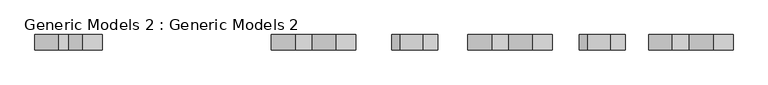
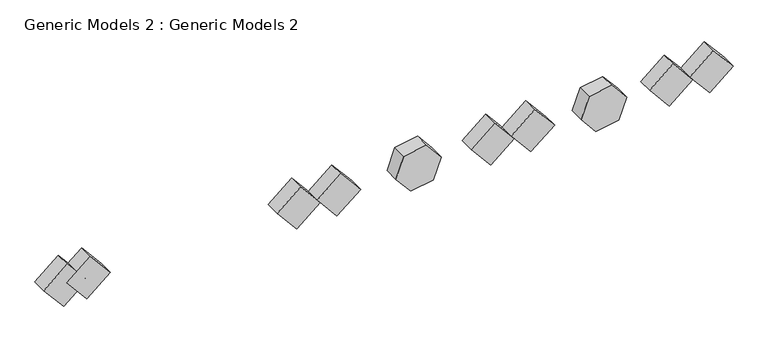
"""IFC4 building model written with IfcOpenShell, lengths in millimetres: proxy geometry, Generic Models 2 : Generic Models 2."""

from ifc_helpers import new_model, si_unit, frame, origin, place, context, project, spatial, polyline, outline, extrude, source, transform, mapped, element, save


def generic_models_2_generic_models_2_4ba01f5b(model_context):
    return source(origin(), model_context, "Body", "SweptSolid", [
        extrude(outline(polyline([(809.5637525, 10146.4778679), (1159.7992719, 9852.5953728), (1080.407325, 9402.3412681), (650.7798588, 9245.9696586), (300.5443394, 9539.8521537), (379.9362862, 9990.1062584), (809.5637525, 10146.4778679)])), frame((0.0, -2288.404596, 0.0), z_axis=(0.0, 1.0, 0.0), x_axis=(0.0, 0.0, 1.0)), (0.0, 0.0, 1.0), 304.8),
        extrude(outline(polyline([(840.3090419, 6475.3232534), (1190.5445612, 6181.4407582), (1111.1526144, 5731.1866535), (681.5251482, 5574.815044), (331.2896288, 5868.6975392), (410.6815756, 6318.9516438), (840.3090419, 6475.3232534)])), frame((0.0, -2288.404596, 0.0), z_axis=(0.0, 1.0, 0.0), x_axis=(0.0, 0.0, 1.0)), (0.0, 0.0, 1.0), 304.8),
        extrude(outline(polyline([(0.0, -609.5999999), (0.0, 0.0), (304.8, 0.0), (304.8, -609.5999999), (0.0, -609.5999999)])), frame((-553.9885527, -2288.404596, 325.3979045), z_axis=(-0.6427876096865387, 0.0, 0.7660444431189787), x_axis=(0.0, 1.0, 0.0)), (0.0, 0.0, 1.0), 609.6),
        extrude(outline(polyline([(0.0, -609.5999999), (0.0, 0.0), (304.8, 0.0), (304.8, -609.5999999), (0.0, -609.5999999)])), frame((-1011.1885527, -2288.404596, 325.3979045), z_axis=(-0.6427876096865386, 0.0, 0.7660444431189787), x_axis=(0.0, 1.0, 0.0)), (0.0, 0.0, 1.0), 609.6),
        extrude(outline(polyline([(0.0, -609.5999999), (0.0, 0.0), (304.8, 0.0), (304.8, -609.5999999), (0.0, -609.5999999)])), frame((11790.4114473, -2288.404596, 325.3979045), z_axis=(-0.6427876096865376, 0.0, 0.7660444431189796), x_axis=(0.0, 1.0, 0.0)), (0.0, 0.0, 1.0), 609.6),
        extrude(outline(polyline([(0.0, -609.5999999), (0.0, 0.0), (304.8, 0.0), (304.8, -609.5999999), (0.0, -609.5999999)])), frame((10994.6351637, -2288.404596, 325.3979045), z_axis=(-0.6427876096865375, 0.0, 0.7660444431189797), x_axis=(0.0, 1.0, 0.0)), (0.0, 0.0, 1.0), 609.6),
        extrude(outline(polyline([(0.0, -609.5999999), (0.0, 0.0), (304.8, 0.0), (304.8, -609.5999999), (0.0, -609.5999999)])), frame((8251.4351637, -2288.404596, 325.3979045), z_axis=(-0.6427876096865383, 0.0, 0.766044443118979), x_axis=(0.0, 1.0, 0.0)), (0.0, 0.0, 1.0), 609.6),
        extrude(outline(polyline([(0.0, -609.5999999), (0.0, 0.0), (304.8, 0.0), (304.8, -609.5999999), (0.0, -609.5999999)])), frame((7455.6588801, -2288.404596, 325.3979045), z_axis=(-0.642787609686538, 0.0, 0.7660444431189792), x_axis=(0.0, 1.0, 0.0)), (0.0, 0.0, 1.0), 609.6),
        extrude(outline(polyline([(0.0, -609.5999999), (0.0, 0.0), (304.8, 0.0), (304.8, -609.5999999), (0.0, -609.5999999)])), frame((4407.6588801, -2288.404596, 325.3979045), z_axis=(-0.6427876096865389, 0.0, 0.7660444431189783), x_axis=(0.0, 1.0, 0.0)), (0.0, 0.0, 1.0), 609.6),
        extrude(outline(polyline([(0.0, -609.6), (0.0, 0.0), (304.8, 0.0), (304.8, -609.6), (0.0, -609.6)])), frame((3611.8825965, -2288.404596, 325.3979045), z_axis=(-0.6427876096865388, 0.0, 0.7660444431189785), x_axis=(0.0, 1.0, 0.0)), (0.0, 0.0, 1.0), 609.6),
    ])


if __name__ == "__main__":
    model = new_model("IFC4")
    model_context = context("Model", 3, world=origin())
    ifc_project = project(units=[si_unit("LENGTHUNIT", "METRE", prefix="MILLI")], contexts=[model_context])
    site = spatial("IfcSite", under=ifc_project)
    building = spatial("IfcBuilding", under=site)
    placement = place(None, origin())
    generic_models_2_generic_models_2_shape = generic_models_2_generic_models_2_4ba01f5b(model_context)
    element("IfcBuildingElementProxy", 1, Name="Generic Models 2 : Generic Models 2", ObjectType="Generic Models 2 : Generic Models 2", at=placement, inside=building, context=model_context, shape_type="MappedRepresentation", body=[
        mapped(generic_models_2_generic_models_2_shape, transform((0.0, 0.0, 0.0), x_axis=(1.0, 0.0, 0.0), y_axis=(0.0, 1.0, 0.0), z_axis=(0.0, 0.0, 1.0))),
    ])
    save(model, "model.ifc")

# Revit data of these elements
# Element 1 (IfcBuildingElementProxy, "Generic Models 2 : Generic Models 2")
#   Materials on its faces: "Cherry", "Clad - White"
# Materials
#   "Cherry": class "Wood", colour RGB 226 177 128, transparency 0, Description = "Prunus Serotina", Cost = 0
#   "Clad - White": class "Wood", colour RGB 242 242 238, transparency 0, Cost = 0
